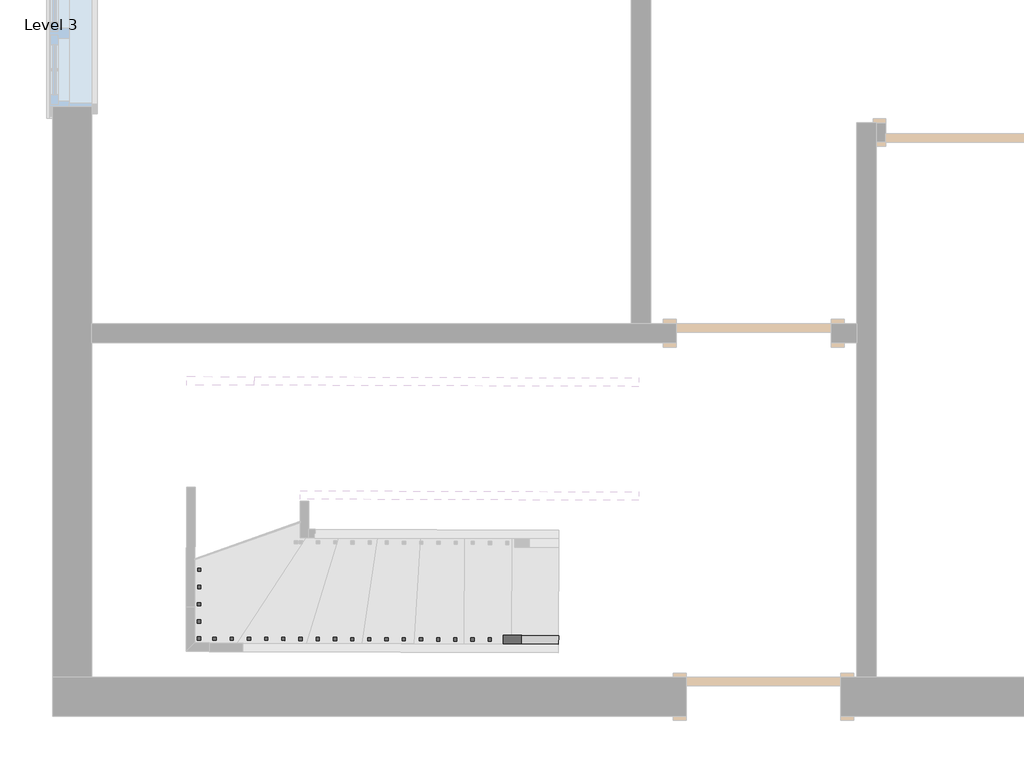
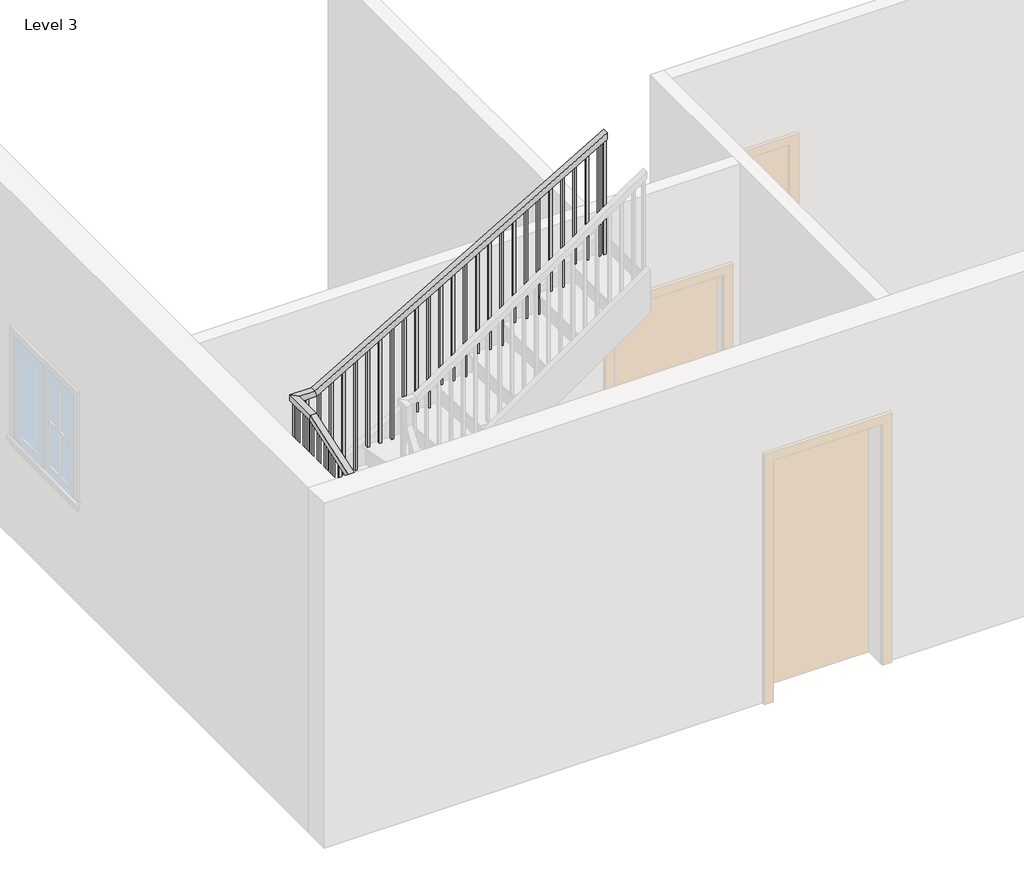
# One storey, part 2 of 3: 1 railing.
"""IFC4 building model written with IfcOpenShell, lengths in millimetres."""

from ifc_helpers import new_model, si_unit, frame, origin, place, context, project, spatial, polyline, outline, extrude, faceted_brep, element, save

model = new_model("IFC4")

# Units and contexts
model_context = context("Model", 3, world=origin())
ifc_project = project(units=[si_unit("LENGTHUNIT", "METRE", prefix="MILLI")], contexts=[model_context])

# Site, building, storey
site = spatial("IfcSite", under=ifc_project)
building = spatial("IfcBuilding", under=site)
storey = spatial("IfcBuildingStorey", under=building, Name="Level 3", Elevation=3200.4)

# Railing
placement = place(None, origin())
element("IfcRailing", 1, ObjectType="Handrail - Rectangular", at=placement, inside=storey, context=model_context, shape_type="SolidModel", body=[
    faceted_brep([(-2342.0274141, -4826.0015756, 4284.1333333), (-2342.0274141, -4826.0015756, 4226.5375993), (-2341.8555281, -4775.2018664, 4226.5375993), (-2341.8555281, -4775.2018664, 4284.1333333), (-4375.5150225, -4819.1210645, 5370.5704289), (-4388.2346185, -4819.0780265, 5319.7704289), (-4388.0627326, -4768.2783173, 5319.7704289), (-4375.3431366, -4768.3213553, 5370.5704289), (-4491.7270905, -4818.7278493, 5370.5704289), (-4491.7270905, -4818.7278493, 5319.7704289), (-4440.7554953, -4768.100026, 5319.7704289), (-4440.7554953, -4768.100026, 5370.5704289), (-4491.153576, -4649.2296115, 5370.5704289), (-4491.1254156, -4640.9069784, 5319.7704289), (-4440.3257064, -4641.0788644, 5319.7704289), (-4440.3538668, -4649.4014974, 5370.5704289), (-4487.5712496, -3590.4977417, 5727.049629), (-4487.5430892, -3582.1751086, 5676.249629), (-4436.74338, -3582.3469946, 5676.249629), (-4436.7715404, -3590.6696276, 5727.049629), (-4486.5726753, -3295.3759891, 5727.049629), (-4486.5726753, -3295.3759891, 5676.249629), (-4435.9448521, -3346.3475843, 5676.249629), (-4435.9448521, -3346.3475843, 5727.049629), (-4306.8228358, -3295.9841909, 5727.049629), (-4292.9867911, -3296.0310065, 5676.249629), (-4293.1586771, -3346.8307157, 5676.249629), (-4306.9947217, -3346.7839001, 5727.049629), (-1866.6470501, -3304.2407725, 7162.8), (-1866.8189361, -3355.0404817, 7162.8), (-1866.8189361, -3355.0404817, 7103.8591495), (-1866.6470501, -3304.2407725, 7103.8591495)], [[[0, 1, 2, 3]], [[1, 0, 4, 5]], [[2, 1, 5, 6]], [[3, 2, 6, 7]], [[0, 3, 7, 4]], [[5, 4, 8, 9]], [[6, 5, 9, 10]], [[7, 6, 10, 11]], [[4, 7, 11, 8]], [[9, 8, 12, 13]], [[10, 9, 13, 14]], [[11, 10, 14, 15]], [[8, 11, 15, 12]], [[13, 12, 16, 17]], [[14, 13, 17, 18]], [[15, 14, 18, 19]], [[12, 15, 19, 16]], [[17, 16, 20, 21]], [[18, 17, 21, 22]], [[19, 18, 22, 23]], [[16, 19, 23, 20]], [[21, 20, 24, 25]], [[22, 21, 25, 26]], [[23, 22, 26, 27]], [[20, 23, 27, 24]], [[28, 29, 30, 31]], [[25, 24, 28, 31]], [[26, 25, 31, 30]], [[27, 26, 30, 29]], [[24, 27, 29, 28]]]),
    extrude(outline(polyline([(234.2042864, 19.05), (1221.3020607, 19.05), (1221.3020607, 0.0), (222.9957135, 0.0), (234.2042864, 19.05)])), frame((-1911.7805866, -3339.0132586, 7300.3687274), z_axis=(0.0033835818014388316, 0.9999942756707125, 0.0), x_axis=(0.0, 0.0, -1.0)), (0.0, 0.0, 1.0), 19.05),
    extrude(outline(polyline([(234.2042864, 19.0499999), (1161.5230057, 19.0499999), (1161.5230057, 0.0), (222.9957136, 0.0), (234.2042864, 19.0499999)])), frame((-2013.3800051, -3338.6694867, 7240.5896724), z_axis=(0.0033835818014388316, 0.9999942756707125, 0.0), x_axis=(0.0, 0.0, -1.0)), (0.0, 0.0, 1.0), 19.05),
    extrude(outline(polyline([(234.2042864, 19.0499999), (1101.7439506, 19.0499999), (1101.7439506, 0.0), (222.9957136, 0.0), (234.2042864, 19.0499999)])), frame((-2114.9794235, -3338.3257147, 7180.8106173), z_axis=(0.0033835818014388316, 0.9999942756707125, 0.0), x_axis=(0.0, 0.0, -1.0)), (0.0, 0.0, 1.0), 19.05),
    extrude(outline(polyline([(234.2042864, 19.0499999), (1211.2982289, 19.0499999), (1211.2982289, 0.0), (222.9957135, 0.0), (234.2042864, 19.0499999)])), frame((-2216.5788419, -3337.9819428, 7121.0315622), z_axis=(0.0033835818014388316, 0.9999942756707125, 0.0), x_axis=(0.0, 0.0, -1.0)), (0.0, 0.0, 1.0), 19.05),
    extrude(outline(polyline([(234.2042864, 19.0499999), (1151.5191739, 19.0499999), (1151.5191739, 0.0), (222.9957136, 0.0), (234.2042864, 19.0499999)])), frame((-2318.1782603, -3337.6381709, 7061.2525072), z_axis=(0.0033835818014388316, 0.9999942756707125, 0.0), x_axis=(0.0, 0.0, -1.0)), (0.0, 0.0, 1.0), 19.05),
    extrude(outline(polyline([(234.2042864, 19.0499999), (1261.0734521, 19.0499999), (1261.0734521, 0.0), (222.9957136, 0.0), (234.2042864, 19.0499999)])), frame((-2419.7776787, -3337.294399, 7001.4734521), z_axis=(0.0033835818014388316, 0.9999942756707125, 0.0), x_axis=(0.0, 0.0, -1.0)), (0.0, 0.0, 1.0), 19.05),
    extrude(outline(polyline([(234.2042864, 19.0499999), (1201.294397, 19.0499999), (1201.294397, 0.0), (222.9957136, 0.0), (234.2042864, 19.0499999)])), frame((-2521.3770971, -3336.9506271, 6941.694397), z_axis=(0.0033835818014388316, 0.9999942756707125, 0.0), x_axis=(0.0, 0.0, -1.0)), (0.0, 0.0, 1.0), 19.05),
    extrude(outline(polyline([(234.2042864, 19.05), (1141.515342, 19.05), (1141.515342, 0.0), (222.9957136, 0.0), (234.2042864, 19.05)])), frame((-2622.9765155, -3336.6068552, 6881.915342), z_axis=(0.0033835818014388316, 0.9999942756707125, 0.0), x_axis=(0.0, 0.0, -1.0)), (0.0, 0.0, 1.0), 19.05),
    extrude(outline(polyline([(234.2042864, 19.05), (1251.0696202, 19.05), (1251.0696202, 0.0), (222.9957136, 0.0), (234.2042864, 19.05)])), frame((-2724.5759339, -3336.2630833, 6822.1362869), z_axis=(0.0033835818014388316, 0.9999942756707125, 0.0), x_axis=(0.0, 0.0, -1.0)), (0.0, 0.0, 1.0), 19.05),
    extrude(outline(polyline([(234.2042864, 19.05), (1191.2905651, 19.05), (1191.2905651, 0.0), (222.9957136, 0.0), (234.2042864, 19.05)])), frame((-2826.1753523, -3335.9193114, 6762.3572318), z_axis=(0.0033835818014388316, 0.9999942756707125, 0.0), x_axis=(0.0, 0.0, -1.0)), (0.0, 0.0, 1.0), 19.05),
    extrude(outline(polyline([(234.2042865, 19.05), (1131.5115101, 19.05), (1131.5115101, 0.0), (222.9957136, 0.0), (234.2042865, 19.05)])), frame((-2927.7747707, -3335.5755395, 6702.5781768), z_axis=(0.0033835818014388316, 0.9999942756707125, 0.0), x_axis=(0.0, 0.0, -1.0)), (0.0, 0.0, 1.0), 19.05),
    extrude(outline(polyline([(234.2042864, 19.05), (1241.0657884, 19.05), (1241.0657884, 0.0), (222.9957136, 0.0), (234.2042864, 19.05)])), frame((-3029.3741891, -3335.2317675, 6642.7991217), z_axis=(0.0033835818014388316, 0.9999942756707125, 0.0), x_axis=(0.0, 0.0, -1.0)), (0.0, 0.0, 1.0), 19.05),
    extrude(outline(polyline([(234.2042864, 19.05), (1181.2867333, 19.05), (1181.2867333, 0.0), (222.9957136, 0.0), (234.2042864, 19.05)])), frame((-3130.9736075, -3334.8879956, 6583.0200666), z_axis=(0.0033835818014388316, 0.9999942756707125, 0.0), x_axis=(0.0, 0.0, -1.0)), (0.0, 0.0, 1.0), 19.05),
    extrude(outline(polyline([(234.2042865, 19.0499999), (1121.5076783, 19.0499999), (1121.5076783, 0.0), (222.9957136, 0.0), (234.2042865, 19.0499999)])), frame((-3232.573026, -3334.5442237, 6523.2410116), z_axis=(0.0033835818014388316, 0.9999942756707125, 0.0), x_axis=(0.0, 0.0, -1.0)), (0.0, 0.0, 1.0), 19.05),
    extrude(outline(polyline([(234.2042864, 19.0499999), (1231.0619565, 19.0499999), (1231.0619565, 0.0), (222.9957136, 0.0), (234.2042864, 19.0499999)])), frame((-3334.1724444, -3334.2004518, 6463.4619565), z_axis=(0.0033835818014388316, 0.9999942756707125, 0.0), x_axis=(0.0, 0.0, -1.0)), (0.0, 0.0, 1.0), 19.05),
    extrude(outline(polyline([(234.2042864, 19.0499999), (1171.2829014, 19.0499999), (1171.2829014, 0.0), (222.9957136, 0.0), (234.2042864, 19.0499999)])), frame((-3435.7718628, -3333.8566799, 6403.6829014), z_axis=(0.0033835818014388316, 0.9999942756707125, 0.0), x_axis=(0.0, 0.0, -1.0)), (0.0, 0.0, 1.0), 19.05),
    extrude(outline(polyline([(234.2042864, 19.0499999), (1111.5038463, 19.0499999), (1111.5038463, 0.0), (222.9957135, 0.0), (234.2042864, 19.0499999)])), frame((-3537.3712812, -3333.512908, 6343.9038463), z_axis=(0.0033835818014388316, 0.9999942756707125, 0.0), x_axis=(0.0, 0.0, -1.0)), (0.0, 0.0, 1.0), 19.05),
    extrude(outline(polyline([(234.2042864, 19.0499999), (1221.0581246, 19.0499999), (1221.0581246, 0.0), (222.9957136, 0.0), (234.2042864, 19.0499999)])), frame((-3638.9706996, -3333.1691361, 6284.1247913), z_axis=(0.0033835818014388316, 0.9999942756707125, 0.0), x_axis=(0.0, 0.0, -1.0)), (0.0, 0.0, 1.0), 19.05),
    extrude(outline(polyline([(234.2042864, 19.0499999), (1161.2790695, 19.0499999), (1161.2790695, 0.0), (222.9957136, 0.0), (234.2042864, 19.0499999)])), frame((-3740.570118, -3332.8253642, 6224.3457362), z_axis=(0.0033835818014388316, 0.9999942756707125, 0.0), x_axis=(0.0, 0.0, -1.0)), (0.0, 0.0, 1.0), 19.05),
    extrude(outline(polyline([(234.2042864, 19.05), (1101.5000144, 19.05), (1101.5000144, 0.0), (222.9957135, 0.0), (234.2042864, 19.05)])), frame((-3842.1695364, -3332.4815923, 6164.5666811), z_axis=(0.0033835818014388316, 0.9999942756707125, 0.0), x_axis=(0.0, 0.0, -1.0)), (0.0, 0.0, 1.0), 19.05),
    extrude(outline(polyline([(234.2042864, 19.05), (1211.0542928, 19.05), (1211.0542928, 0.0), (222.9957136, 0.0), (234.2042864, 19.05)])), frame((-3943.7689548, -3332.1378203, 6104.7876261), z_axis=(0.0033835818014388316, 0.9999942756707125, 0.0), x_axis=(0.0, 0.0, -1.0)), (0.0, 0.0, 1.0), 19.05),
    extrude(outline(polyline([(234.2042864, 19.05), (1151.2752377, 19.05), (1151.2752377, 0.0), (222.9957136, 0.0), (234.2042864, 19.05)])), frame((-4045.3683732, -3331.7940484, 6045.008571), z_axis=(0.0033835818014388316, 0.9999942756707125, 0.0), x_axis=(0.0, 0.0, -1.0)), (0.0, 0.0, 1.0), 19.05),
    extrude(outline(polyline([(234.2042864, 19.05), (1091.4961826, 19.05), (1091.4961826, 0.0), (222.9957136, 0.0), (234.2042864, 19.05)])), frame((-4146.9677916, -3331.4502765, 5985.2295159), z_axis=(0.0033835818014388316, 0.9999942756707125, 0.0), x_axis=(0.0, 0.0, -1.0)), (0.0, 0.0, 1.0), 19.05),
    extrude(outline(polyline([(234.2042865, 19.05), (1031.7171276, 19.05), (1031.7171276, 0.0), (222.9957136, 0.0), (234.2042865, 19.05)])), frame((-4248.56721, -3331.1065046, 5925.4504609), z_axis=(0.0033835818014388316, 0.9999942756707125, 0.0), x_axis=(0.0, 0.0, -1.0)), (0.0, 0.0, 1.0), 19.05),
    extrude(outline(polyline([(-4369.1520622, -3311.6483845), (-4350.1021712, -3311.7128418), (-4350.1666284, -3330.7627327), (-4369.2165194, -3330.6982755), (-4369.1520622, -3311.6483845)])), frame((0.0, 0.0, 4893.7333333), z_axis=(0.0, 0.0, 1.0), x_axis=(1.0, 0.0, 0.0)), (0.0, 0.0, 1.0), 782.5162957),
    extrude(outline(polyline([(-4470.9856602, -3380.5147968), (-4470.921203, -3361.4649058), (-4451.871312, -3361.5293631), (-4451.9357693, -3380.579254), (-4470.9856602, -3380.5147968)])), frame((0.0, 0.0, 4893.7333333), z_axis=(0.0, 0.0, 1.0), x_axis=(1.0, 0.0, 0.0)), (0.0, 0.0, 1.0), 782.5162957),
    extrude(outline(polyline([(-4471.3294321, -3482.1142152), (-4471.2649749, -3463.0643242), (-4452.215084, -3463.1287815), (-4452.2795412, -3482.1786724), (-4471.3294321, -3482.1142152)])), frame((0.0, 0.0, 4724.4), z_axis=(0.0, 0.0, 1.0), x_axis=(1.0, 0.0, 0.0)), (0.0, 0.0, 1.0), 951.849629),
    extrude(outline(polyline([(-4471.6732041, -3583.7136336), (-4471.6087468, -3564.6637426), (-4452.5588559, -3564.7281999), (-4452.6233131, -3583.7780908), (-4471.6732041, -3583.7136336)])), frame((0.0, 0.0, 4724.4), z_axis=(0.0, 0.0, 1.0), x_axis=(1.0, 0.0, 0.0)), (0.0, 0.0, 1.0), 951.849629),
    extrude(outline(polyline([(231.8070867, 19.0499999), (1148.9478489, 19.0499999), (1148.9478489, 0.0), (225.3929132, 0.0), (231.8070867, 19.0499999)])), frame((-4452.9026278, -3666.3276183, 5873.3478489), z_axis=(-0.9999942756707125, 0.003383581801438912, 0.0), x_axis=(0.0, 0.0, -1.0)), (0.0, 0.0, 1.0), 19.05),
    extrude(outline(polyline([(231.8070868, 19.0499999), (1114.7389237, 19.0499999), (1114.7389237, 0.0), (225.3929133, 0.0), (231.8070868, 19.0499999)])), frame((-4453.2463997, -3767.9270367, 5839.1389237), z_axis=(-0.9999942756707125, 0.003383581801438912, 0.0), x_axis=(0.0, 0.0, -1.0)), (0.0, 0.0, 1.0), 19.05),
    extrude(outline(polyline([(231.8070867, 19.0499999), (1080.5299984, 19.0499999), (1080.5299984, 0.0), (225.3929132, 0.0), (231.8070867, 19.0499999)])), frame((-4453.5901716, -3869.5264551, 5804.9299984), z_axis=(-0.9999942756707125, 0.003383581801438912, 0.0), x_axis=(0.0, 0.0, -1.0)), (0.0, 0.0, 1.0), 19.05),
    extrude(outline(polyline([(231.8070867, 19.05), (1215.6544064, 19.05), (1215.6544064, 0.0), (225.3929132, 0.0), (231.8070867, 19.05)])), frame((-4453.9339435, -3971.1258735, 5770.7210731), z_axis=(-0.9999942756707125, 0.003383581801438912, 0.0), x_axis=(0.0, 0.0, -1.0)), (0.0, 0.0, 1.0), 19.05),
    extrude(outline(polyline([(231.8070868, 19.05), (1181.4454812, 19.05), (1181.4454812, 0.0), (225.3929133, 0.0), (231.8070868, 19.05)])), frame((-4454.2777154, -4072.7252919, 5736.5121479), z_axis=(-0.9999942756707125, 0.003383581801438912, 0.0), x_axis=(0.0, 0.0, -1.0)), (0.0, 0.0, 1.0), 19.05),
    extrude(outline(polyline([(231.8070867, 19.05), (1147.2365559, 19.05), (1147.2365559, 0.0), (225.3929132, 0.0), (231.8070867, 19.05)])), frame((-4454.6214873, -4174.3247103, 5702.3032226), z_axis=(-0.9999942756707125, 0.003383581801438912, 0.0), x_axis=(0.0, 0.0, -1.0)), (0.0, 0.0, 1.0), 19.05),
    extrude(outline(polyline([(231.8070868, 19.05), (1113.0276307, 19.05), (1113.0276307, 0.0), (225.3929133, 0.0), (231.8070868, 19.05)])), frame((-4454.9652592, -4275.9241287, 5668.0942974), z_axis=(-0.9999942756707125, 0.003383581801438912, 0.0), x_axis=(0.0, 0.0, -1.0)), (0.0, 0.0, 1.0), 19.05),
    extrude(outline(polyline([(231.8070868, 19.05), (1248.1520388, 19.05), (1248.1520388, 0.0), (225.3929133, 0.0), (231.8070868, 19.05)])), frame((-4455.3090312, -4377.5235471, 5633.8853721), z_axis=(-0.9999942756707125, 0.003383581801438912, 0.0), x_axis=(0.0, 0.0, -1.0)), (0.0, 0.0, 1.0), 19.05),
    extrude(outline(polyline([(231.8070867, 19.05), (1213.9431135, 19.05), (1213.9431135, 0.0), (225.3929132, 0.0), (231.8070867, 19.05)])), frame((-4455.6528031, -4479.1229655, 5599.6764468), z_axis=(-0.9999942756707125, 0.003383581801438912, 0.0), x_axis=(0.0, 0.0, -1.0)), (0.0, 0.0, 1.0), 19.05),
    extrude(outline(polyline([(231.8070868, 19.0499999), (1179.7341883, 19.0499999), (1179.7341883, 0.0), (225.3929133, 0.0), (231.8070868, 19.0499999)])), frame((-4455.996575, -4580.722384, 5565.4675216), z_axis=(-0.9999942756707125, 0.003383581801438912, 0.0), x_axis=(0.0, 0.0, -1.0)), (0.0, 0.0, 1.0), 19.05),
    extrude(outline(polyline([(-4475.4546951, -4701.3072361), (-4475.3902378, -4682.2573451), (-4456.3403469, -4682.3218024), (-4456.4048041, -4701.3716933), (-4475.4546951, -4701.3072361)])), frame((0.0, 0.0, 4385.7333333), z_axis=(0.0, 0.0, 1.0), x_axis=(1.0, 0.0, 0.0)), (0.0, 0.0, 1.0), 934.0370956),
    extrude(outline(polyline([(223.5110808, 19.05), (1155.0403583, 19.05), (1155.0403583, 0.0), (233.6889192, 0.0), (223.5110808, 19.05)])), frame((-4364.4371224, -4803.2834569, 5540.7736916), z_axis=(0.0033835818014387046, 0.9999942756707125, 0.0), x_axis=(0.0, 0.0, -1.0)), (0.0, 0.0, 1.0), 19.05),
    extrude(outline(polyline([(223.5110808, 19.05), (1100.7585537, 19.05), (1100.7585537, 0.0), (233.6889192, 0.0), (223.5110808, 19.05)])), frame((-4262.837704, -4803.6272288, 5486.491887), z_axis=(0.0033835818014387046, 0.9999942756707125, 0.0), x_axis=(0.0, 0.0, -1.0)), (0.0, 0.0, 1.0), 19.05),
    extrude(outline(polyline([(223.5110808, 19.05), (1215.8100824, 19.05), (1215.8100824, 0.0), (233.6889192, 0.0), (223.5110808, 19.05)])), frame((-4161.2382856, -4803.9710007, 5432.2100824), z_axis=(0.0033835818014387046, 0.9999942756707125, 0.0), x_axis=(0.0, 0.0, -1.0)), (0.0, 0.0, 1.0), 19.05),
    extrude(outline(polyline([(223.5110809, 19.0499999), (1161.5282778, 19.0499999), (1161.5282778, 0.0), (233.6889192, 0.0), (223.5110809, 19.0499999)])), frame((-4059.6388672, -4804.3147726, 5377.9282778), z_axis=(0.0033835818014387046, 0.9999942756707125, 0.0), x_axis=(0.0, 0.0, -1.0)), (0.0, 0.0, 1.0), 19.05),
    extrude(outline(polyline([(223.5110808, 19.0499999), (1107.2464731, 19.0499999), (1107.2464731, 0.0), (233.6889191, 0.0), (223.5110808, 19.0499999)])), frame((-3958.0394488, -4804.6585445, 5323.6464731), z_axis=(0.0033835818014387046, 0.9999942756707125, 0.0), x_axis=(0.0, 0.0, -1.0)), (0.0, 0.0, 1.0), 19.05),
    extrude(outline(polyline([(223.5110808, 19.0499999), (1052.9646685, 19.0499999), (1052.9646685, 0.0), (233.6889192, 0.0), (223.5110808, 19.0499999)])), frame((-3856.4400304, -4805.0023164, 5269.3646685), z_axis=(0.0033835818014387046, 0.9999942756707125, 0.0), x_axis=(0.0, 0.0, -1.0)), (0.0, 0.0, 1.0), 19.05),
    extrude(outline(polyline([(223.5110808, 19.0499999), (1168.0161972, 19.0499999), (1168.0161972, 0.0), (233.6889192, 0.0), (223.5110808, 19.0499999)])), frame((-3754.840612, -4805.3460883, 5215.0828639), z_axis=(0.0033835818014387046, 0.9999942756707125, 0.0), x_axis=(0.0, 0.0, -1.0)), (0.0, 0.0, 1.0), 19.05),
    extrude(outline(polyline([(223.5110808, 19.0499999), (1113.7343926, 19.0499999), (1113.7343926, 0.0), (233.6889192, 0.0), (223.5110808, 19.0499999)])), frame((-3653.2411936, -4805.6898602, 5160.8010593), z_axis=(0.0033835818014387046, 0.9999942756707125, 0.0), x_axis=(0.0, 0.0, -1.0)), (0.0, 0.0, 1.0), 19.05),
    extrude(outline(polyline([(223.5110808, 19.0499999), (1059.452588, 19.0499999), (1059.452588, 0.0), (233.6889192, 0.0), (223.5110808, 19.0499999)])), frame((-3551.6417752, -4806.0336322, 5106.5192547), z_axis=(0.0033835818014387046, 0.9999942756707125, 0.0), x_axis=(0.0, 0.0, -1.0)), (0.0, 0.0, 1.0), 19.05),
    extrude(outline(polyline([(223.5110808, 19.05), (1174.5041168, 19.05), (1174.5041168, 0.0), (233.6889192, 0.0), (223.5110808, 19.05)])), frame((-3450.0423567, -4806.3774041, 5052.2374501), z_axis=(0.0033835818014387046, 0.9999942756707125, 0.0), x_axis=(0.0, 0.0, -1.0)), (0.0, 0.0, 1.0), 19.05),
    extrude(outline(polyline([(223.5110809, 19.05), (1120.2223122, 19.05), (1120.2223122, 0.0), (233.6889192, 0.0), (223.5110809, 19.05)])), frame((-3348.4429383, -4806.721176, 4997.9556455), z_axis=(0.0033835818014387046, 0.9999942756707125, 0.0), x_axis=(0.0, 0.0, -1.0)), (0.0, 0.0, 1.0), 19.05),
    extrude(outline(polyline([(223.5110808, 19.05), (1065.9405075, 19.05), (1065.9405075, 0.0), (233.6889191, 0.0), (223.5110808, 19.05)])), frame((-3246.8435199, -4807.0649479, 4943.6738408), z_axis=(0.0033835818014387046, 0.9999942756707125, 0.0), x_axis=(0.0, 0.0, -1.0)), (0.0, 0.0, 1.0), 19.05),
    extrude(outline(polyline([(223.5110808, 19.05), (1180.9920362, 19.05), (1180.9920362, 0.0), (233.6889192, 0.0), (223.5110808, 19.05)])), frame((-3145.2441015, -4807.4087198, 4889.3920362), z_axis=(0.0033835818014387046, 0.9999942756707125, 0.0), x_axis=(0.0, 0.0, -1.0)), (0.0, 0.0, 1.0), 19.05),
    extrude(outline(polyline([(223.5110808, 19.05), (1126.7102316, 19.05), (1126.7102316, 0.0), (233.6889192, 0.0), (223.5110808, 19.05)])), frame((-3043.6446831, -4807.7524917, 4835.1102316), z_axis=(0.0033835818014387046, 0.9999942756707125, 0.0), x_axis=(0.0, 0.0, -1.0)), (0.0, 0.0, 1.0), 19.05),
    extrude(outline(polyline([(223.5110808, 19.05), (1072.428427, 19.05), (1072.428427, 0.0), (233.6889192, 0.0), (223.5110808, 19.05)])), frame((-2942.0452647, -4808.0962636, 4780.828427), z_axis=(0.0033835818014387046, 0.9999942756707125, 0.0), x_axis=(0.0, 0.0, -1.0)), (0.0, 0.0, 1.0), 19.05),
    extrude(outline(polyline([(223.5110808, 19.05), (1187.4799557, 19.05), (1187.4799557, 0.0), (233.6889192, 0.0), (223.5110808, 19.05)])), frame((-2840.4458463, -4808.4400355, 4726.5466224), z_axis=(0.0033835818014387046, 0.9999942756707125, 0.0), x_axis=(0.0, 0.0, -1.0)), (0.0, 0.0, 1.0), 19.05),
    extrude(outline(polyline([(223.5110809, 19.0499999), (1133.1981511, 19.0499999), (1133.1981511, 0.0), (233.6889192, 0.0), (223.5110809, 19.0499999)])), frame((-2738.8464279, -4808.7838074, 4672.2648178), z_axis=(0.0033835818014387046, 0.9999942756707125, 0.0), x_axis=(0.0, 0.0, -1.0)), (0.0, 0.0, 1.0), 19.05),
    extrude(outline(polyline([(223.5110809, 19.0499999), (1078.9163465, 19.0499999), (1078.9163465, 0.0), (233.6889192, 0.0), (223.5110809, 19.0499999)])), frame((-2637.2470095, -4809.1275794, 4617.9830132), z_axis=(0.0033835818014387046, 0.9999942756707125, 0.0), x_axis=(0.0, 0.0, -1.0)), (0.0, 0.0, 1.0), 19.05),
    extrude(outline(polyline([(223.5110808, 19.0499999), (1193.9678752, 19.0499999), (1193.9678752, 0.0), (233.6889191, 0.0), (223.5110808, 19.0499999)])), frame((-2535.6475911, -4809.4713513, 4563.7012085), z_axis=(0.0033835818014387046, 0.9999942756707125, 0.0), x_axis=(0.0, 0.0, -1.0)), (0.0, 0.0, 1.0), 19.05),
    extrude(outline(polyline([(223.5110808, 19.0499999), (1139.6860706, 19.0499999), (1139.6860706, 0.0), (233.6889192, 0.0), (223.5110808, 19.0499999)])), frame((-2434.0481727, -4809.8151232, 4509.4194039), z_axis=(0.0033835818014387046, 0.9999942756707125, 0.0), x_axis=(0.0, 0.0, -1.0)), (0.0, 0.0, 1.0), 19.05),
    extrude(outline(polyline([(-4470.8159378, -3330.3545036), (-4470.7514806, -3311.3046126), (-4451.7015896, -3311.3690698), (-4451.7660469, -3330.4189608), (-4470.8159378, -3330.3545036)])), frame((0.0, 0.0, 4893.7333333), z_axis=(0.0, 0.0, 1.0), x_axis=(1.0, 0.0, 0.0)), (0.0, 0.0, 1.0), 782.5162957),
    extrude(outline(polyline([(-4456.748576, -4802.9711117), (-4475.798467, -4802.9066545), (-4475.7340098, -4783.8567635), (-4456.6841188, -4783.9212208), (-4456.748576, -4802.9711117)])), frame((0.0, 0.0, 4385.7333333), z_axis=(0.0, 0.0, 1.0), x_axis=(1.0, 0.0, 0.0)), (0.0, 0.0, 1.0), 934.0370956),
    extrude(outline(polyline([(234.2042864, 19.05), (1247.7881964, 19.05), (1247.7881964, 0.0), (222.9957136, 0.0), (234.2042864, 19.05)])), frame((-1866.7652217, -3339.1655726, 7326.8548631), z_axis=(0.0033835818014388316, 0.9999942756707125, 0.0), x_axis=(0.0, 0.0, -1.0)), (0.0, 0.0, 1.0), 19.05),
    extrude(outline(polyline([(223.5110808, 19.05), (1090.4931852, 19.05), (1090.4931852, 0.0), (233.6889192, 0.0), (223.5110808, 19.05)])), frame((-2341.9736997, -4810.1266665, 4460.2265185), z_axis=(0.0033835818014387046, 0.9999942756707125, 0.0), x_axis=(0.0, 0.0, -1.0)), (0.0, 0.0, 1.0), 19.05),
])

save(model, "model.ifc")

# Revit data of these elements
# Type "Handrail - Rectangular"
#   Assembly Code = "C2010400"
#   built-in parameter 1008612 = 0.0416667 (stored number, unit not read)
#   built-in parameter 1008611 = 0.0416667 (stored number, unit not read)
#   built-in parameter 1008609 = 0.333333 (stored number, unit not read)
#   built-in parameter 1008604 = 0.166667 (stored number, unit not read)
#   built-in parameter 1008603 = 0.166667 (stored number, unit not read)
#   Railing Height = 3' - 0"
#   built-in parameter 1008630 = 2
#   built-in parameter 1008610 = 2
#   built-in parameter 1008618 = Baluster - Square : 3/4"
# Element 1 (IfcRailing, "Handrail - Rectangular")
#   Phase Created = New Construction
